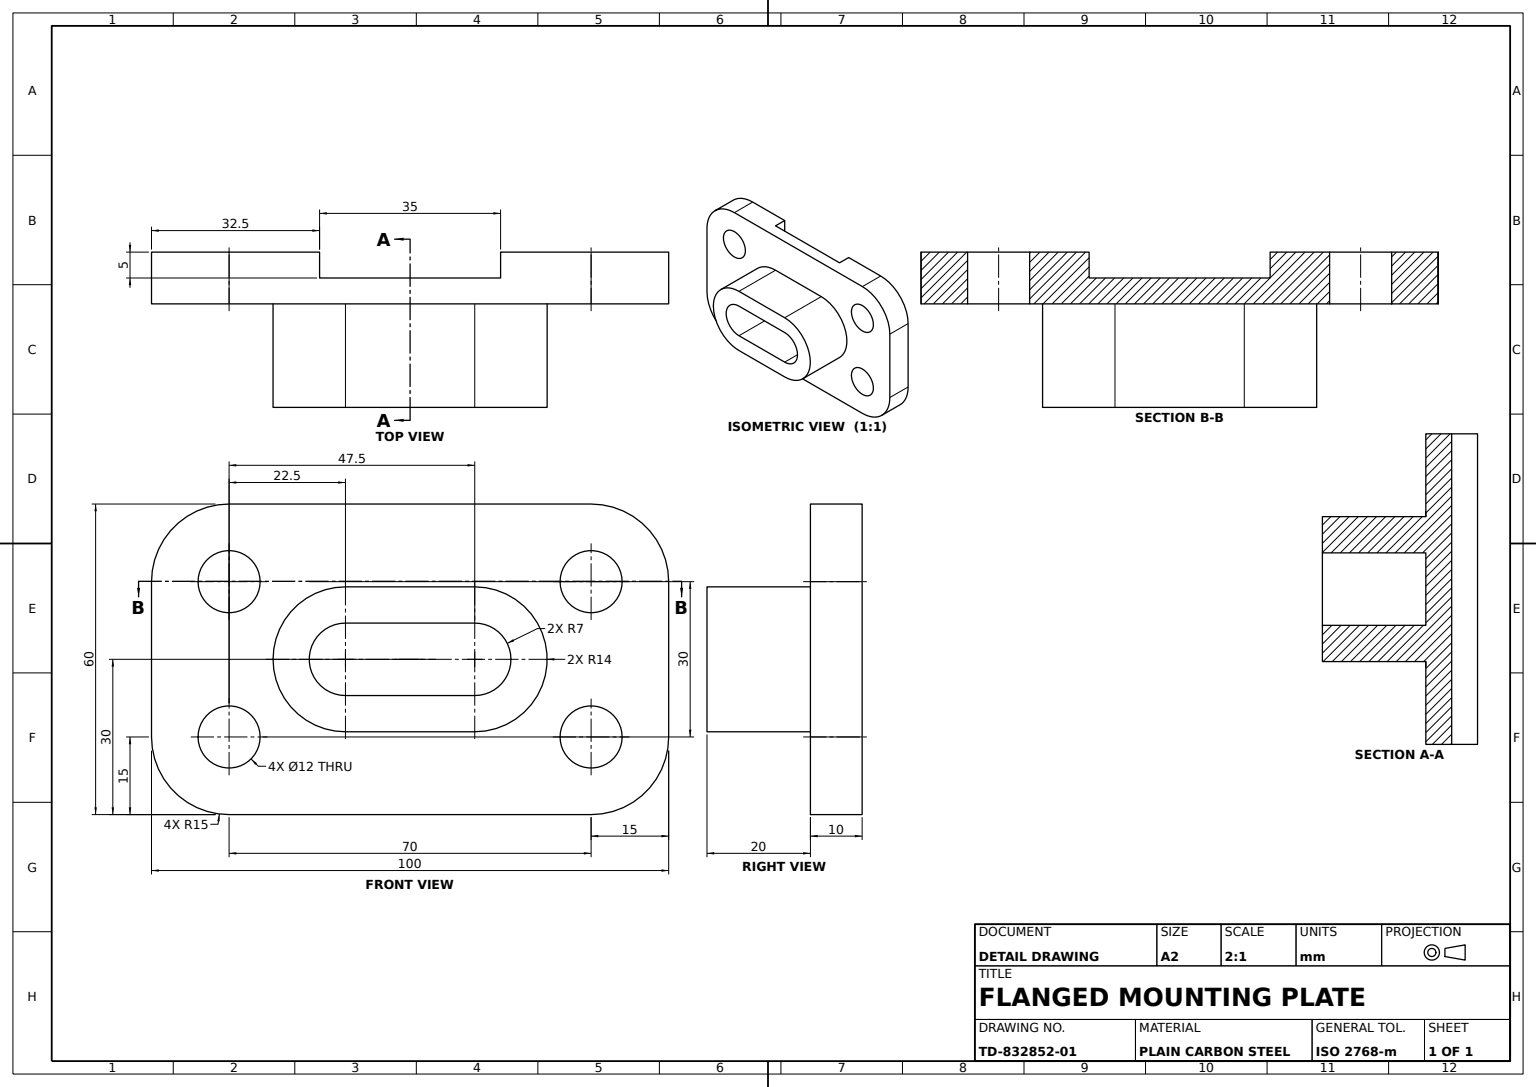
SolidWorks part; units mm, degrees
material "Plain Carbon Steel"
ref_plane "Front Plane" through (0, 0, 0) normal (0, 0, 1) x (1, 0, 0)
ref_plane "Top Plane" through (0, 0, 0) normal (0, 1, 0) x (1, 0, 0)
ref_plane "Right Plane" through (0, 0, 0) normal (1, 0, 0) x (0, 0, -1)
sketch "Base Plate Sketch" plane through (0, 0, 0) normal (0, 0, 1) x (1, 0, 0)
  line L0 (15, 0) -> (85, 0)
  line L1 (100, -15) -> (100, -45)
  line L2 (85, -60) -> (15, -60)
  line L3 (0, -45) -> (0, -15)
  arc A0 (15, -60) -> (0, -45) centre (15, -45) cw
  arc A1 (85, -60) -> (100, -45) centre (85, -45) ccw
  arc A2 (100, -15) -> (85, 0) centre (85, -15) ccw
  arc A3 (15, 0) -> (0, -15) centre (15, -15) ccw
  point P13 (0, 0)
  dimension "D1" = 15
  dimension "D3" = 15
  dimension "D2" = 30
  dimension "D4" = 70
extrude "Base Plate" add sketch "Base Plate Sketch" along normal blind 10
sketch "Mounting Holes Sketch" plane through (0, 0, 10) normal (0, 0, 1) x (1, 0, 0)
  line L0 (0, -15) -> (0, -45) construction
  line L1 (85, 0) -> (15, 0) construction
  circle A0 centre (15, -15) radius 6
  circle A1 centre (85, -15) radius 6
  circle A2 centre (85, -45) radius 6
  circle A3 centre (15, -45) radius 6
  dimension "D1" = 12
  dimension "D4" = 12
  dimension "D5" = 12
  dimension "D6" = 12
  dimension "D7" = 12
  dimension "D8" = 12
  dimension "D9" = 12
  dimension "D10" = 12
  dimension "D2" = 15
  dimension "D3" = 15
extrude "Mounting Holes 4x" cut sketch "Mounting Holes Sketch" against normal blind 10
sketch "Slot Boss Sketch" plane through (0, 0, 10) normal (0, 0, 1) x (1, 0, 0)
  line L0 (15, -60) -> (85, -60) construction
  line L2 (37.5, -16) -> (62.5, -16)
  line L4 (62.5, -44) -> (37.5, -44)
  arc A0 (62.5, -44) -> (62.5, -16) centre (62.5, -30) ccw
  arc A1 (37.5, -16) -> (37.5, -44) centre (37.5, -30) ccw
  dimension "D1" = 14
  dimension "D2" = 22.5
  dimension "D3" = 47.5
  dimension "D4" = 30
extrude "Slot Boss" add sketch "Slot Boss Sketch" along normal blind 20
sketch "Slot Cut Sketch" plane through (0, 0, 30) normal (0, 0, 1) x (1, 0, 0)
  line L0 (37.5, -23) -> (62.5, -23)
  line L2 (62.5, -37) -> (37.5, -37)
  arc A0 (37.5, -23) -> (37.5, -37) centre (37.5, -30) ccw
  arc A1 (62.5, -37) -> (62.5, -23) centre (62.5, -30) ccw
extrude "Slot Through Cut" cut sketch "Slot Cut Sketch" against normal blind 20
sketch "Back Channel Sketch" plane through (0, -60, 0) normal (0, -1, 0) x (1, 0, 0)
  line L0 (50, 0) -> (67.5, 0)
  line L1 (15, 0) -> (85, 0) construction
  line L2 (67.5, 0) -> (67.5, 5)
  line L3 (67.5, 5) -> (32.5, 5)
  line L4 (32.5, 5) -> (32.5, 0)
  line L5 (32.5, 0) -> (50, 0)
  line L6 (85, 10) -> (85, 0) construction
  dimension "D1" = 17.5
  dimension "D2" = 5
extrude "Back Channel Cut" cut sketch "Back Channel Sketch" against normal blind 60
